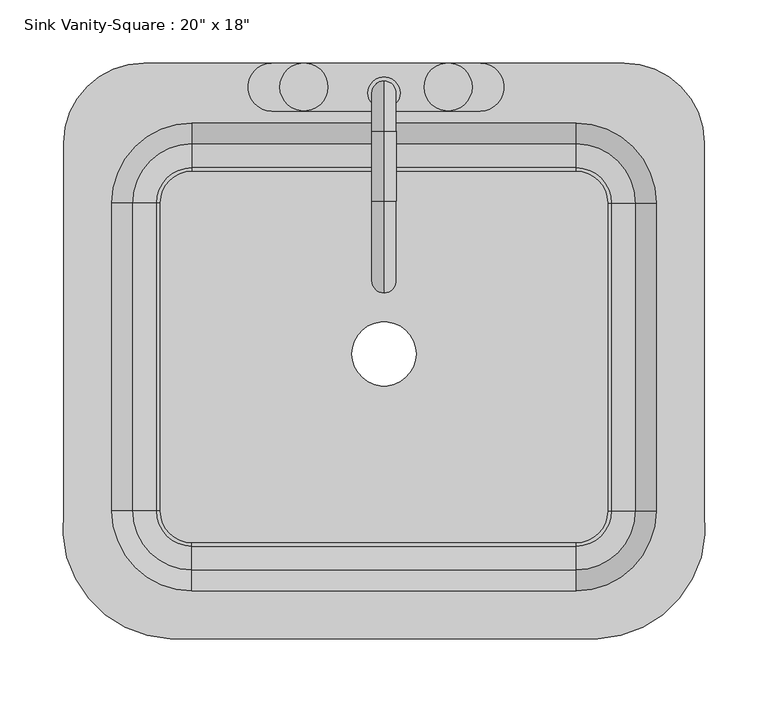
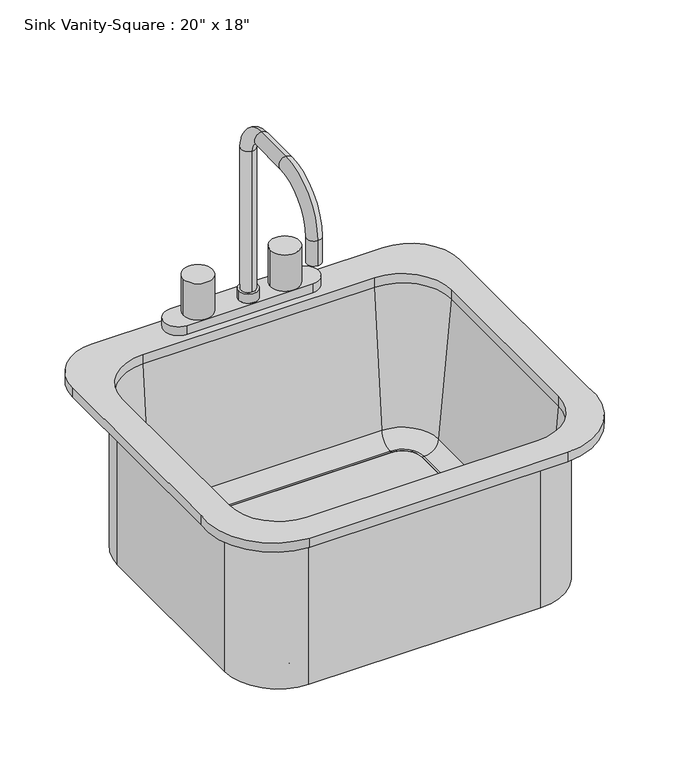
"""IFC4 building model written with IfcOpenShell, lengths in millimetres: flow terminal geometry."""

from ifc_helpers import new_model, si_unit, point, frame, frame_2d, origin, place, context, project, spatial, polyline, circle_curve, ellipse_curve, trimmed, segment, composite_curve, outline, extrude, source, transform, mapped, element, save
from ifc_brep_helpers import plane_surface, cylinder_surface, revolved_surface, advanced_brep


def flow_terminal_62a433f7(model_context):
    return source(origin(), model_context, "Body", "SolidModel", [
        advanced_brep(
        [(-153.9606923, -277.0545989, 800.1), (185.3391735, -277.0545989, 800.1), (269.6892406, -175.4545989, 800.1), (269.6892406, 116.6454011, 800.1), (206.1892406, 180.1454011, 800.1), (-174.8107593, 180.1454011, 800.1), (-238.3107593, 116.6454011, 800.1), (-238.3107593, -175.4545982, 800.1), (168.0892406, 132.5204011, 800.1), (231.5892406, 69.0204011, 800.1), (231.5892406, -175.4545989, 800.1), (168.0892406, -238.9545989, 800.1), (-136.7107594, -238.9545989, 800.1), (-200.2107594, -175.4545989, 800.1), (-200.2107594, 69.0204011, 800.1), (-136.7107594, 132.5204011, 800.1), (-153.9606923, -277.0545989, 787.4), (-238.3107593, -175.4545982, 787.4), (-238.3107593, 116.6454011, 787.4), (-174.8107593, 180.1454011, 787.4), (206.1892406, 180.1454011, 787.4), (269.6892406, 116.6454011, 787.4), (269.6892406, -175.4545989, 787.4), (185.3391735, -277.0545989, 787.4), (237.9392406, 69.0204011, 787.4), (168.0892406, 138.8704011, 787.4), (-136.7107594, 138.8704011, 787.4), (-206.5607594, 69.0204011, 787.4), (-206.5607594, -175.4545989, 787.4), (-136.7107594, -245.3045989, 787.4), (168.0892406, -245.3045989, 787.4), (237.9392406, -175.4545989, 787.4), (168.0892406, 132.5204011, 787.4), (231.5892406, 69.0204011, 787.4), (231.5892406, -175.4545989, 787.4), (168.0892406, -238.9545989, 787.4), (-136.7107594, -238.9545989, 787.4), (-200.2107594, -175.4545989, 787.4), (-200.2107594, 69.0204011, 787.4), (-136.7107594, 132.5204011, 787.4), (237.9392406, 69.0204011, 571.5), (168.0892406, 138.8704011, 571.5), (193.4892406, 69.0204011, 571.5), (168.0892406, 94.4204011, 571.5), (193.4892406, 69.0204011, 581.025), (168.0892406, 94.4204011, 581.025), (196.0776588, 69.0204011, 581.025), (168.0892406, 97.0088193, 581.025), (215.0551678, 69.0204011, 598.4146831), (168.0892406, 115.9863283, 598.4146831), (237.9392406, -175.4545989, 571.5), (193.4892406, -175.4545989, 571.5), (193.4892406, -175.4545989, 581.025), (196.0776588, -175.4545989, 581.025), (215.0551678, -175.4545989, 598.4146831), (168.0892406, -245.3045989, 571.5), (168.0892406, -200.8545989, 571.5), (168.0892406, -200.8545989, 581.025), (168.0892406, -203.4430171, 581.025), (168.0892406, -222.4205261, 598.4146831), (-136.7107594, -245.3045989, 571.5), (-136.7107594, -200.8545989, 571.5), (-136.7107594, -200.8545989, 581.025), (-136.7107594, -203.4430171, 581.025), (-136.7107594, -222.4205261, 598.4146831), (-206.5607594, -175.4545989, 571.5), (-162.1107594, -175.4545989, 571.5), (-162.1107594, -175.4545989, 581.025), (-164.6991776, -175.4545989, 581.025), (-183.6766866, -175.4545989, 598.4146831), (-206.5607594, 69.0204011, 571.5), (-162.1107594, 69.0204011, 571.5), (-162.1107594, 69.0204011, 581.025), (-164.6991776, 69.0204011, 581.025), (-183.6766866, 69.0204011, 598.4146831), (-136.7107594, 138.8704011, 571.5), (-136.7107594, 94.4204011, 571.5), (-136.7107594, 94.4204011, 581.025), (-136.7107594, 97.0088193, 581.025), (-136.7107594, 115.9863283, 598.4146831)],
        [
            (0, 1),
            (1, 2, circle_curve(frame((181.5319557, -188.0793432, 800.1), z_axis=(0.0, 0.0, 1.0), x_axis=(1.0, 0.0, 0.0)), 89.0566732)),
            (2, 3),
            (3, 4, circle_curve(frame((206.1892406, 116.6454011, 800.1), z_axis=(0.0, 0.0, 1.0), x_axis=(1.0, 0.0, 0.0)), 63.5)),
            (4, 5),
            (5, 6, circle_curve(frame((-174.8107593, 116.6454011, 800.1), z_axis=(0.0, 0.0, 1.0), x_axis=(1.0, 0.0, 0.0)), 63.5)),
            (6, 7),
            (7, 0, circle_curve(frame((-150.1534746, -188.0793432, 800.1), z_axis=(0.0, 0.0, 1.0), x_axis=(1.0, 0.0, 0.0)), 89.0566732)),
            (8, 9, circle_curve(frame((168.0892406, 69.0204011, 800.1), z_axis=(0.0, 0.0, -1.0), x_axis=(1.0, 0.0, 0.0)), 63.5)),
            (9, 10),
            (10, 11, circle_curve(frame((168.0892406, -175.4545989, 800.1), z_axis=(0.0, 0.0, -1.0), x_axis=(1.0, 0.0, 0.0)), 63.5)),
            (11, 12),
            (12, 13, circle_curve(frame((-136.7107594, -175.4545989, 800.1), z_axis=(0.0, 0.0, -1.0), x_axis=(1.0, 0.0, 0.0)), 63.5)),
            (13, 14),
            (14, 15, circle_curve(frame((-136.7107594, 69.0204011, 800.1), z_axis=(0.0, 0.0, -1.0), x_axis=(1.0, 0.0, 0.0)), 63.5)),
            (15, 8),
            (16, 17, circle_curve(frame((-150.1534746, -188.0793432, 787.4), z_axis=(0.0, 0.0, -1.0), x_axis=(1.0, 0.0, 0.0)), 89.0566732)),
            (17, 18),
            (18, 19, circle_curve(frame((-174.8107593, 116.6454011, 787.4), z_axis=(0.0, 0.0, -1.0), x_axis=(1.0, 0.0, 0.0)), 63.5)),
            (19, 20),
            (20, 21, circle_curve(frame((206.1892406, 116.6454011, 787.4), z_axis=(0.0, 0.0, -1.0), x_axis=(1.0, 0.0, 0.0)), 63.5)),
            (21, 22),
            (22, 23, circle_curve(frame((181.5319557, -188.0793432, 787.4), z_axis=(0.0, 0.0, -1.0), x_axis=(1.0, 0.0, 0.0)), 89.0566732)),
            (23, 16),
            (24, 25, circle_curve(frame((168.0892406, 69.0204011, 787.4), z_axis=(0.0, 0.0, 1.0), x_axis=(0.0, 1.0, 0.0)), 69.85)),
            (25, 26),
            (26, 27, circle_curve(frame((-136.7107594, 69.0204011, 787.4), z_axis=(0.0, 0.0, 1.0), x_axis=(-1.0, 0.0, 0.0)), 69.85)),
            (27, 28),
            (28, 29, circle_curve(frame((-136.7107594, -175.4545989, 787.4), z_axis=(0.0, 0.0, 1.0), x_axis=(0.0, -1.0, 0.0)), 69.85)),
            (29, 30),
            (30, 31, circle_curve(frame((168.0892406, -175.4545989, 787.4), z_axis=(0.0, 0.0, 1.0), x_axis=(1.0, 0.0, 0.0)), 69.85)),
            (31, 24),
            (0, 16),
            (23, 1),
            (22, 2),
            (21, 3),
            (20, 4),
            (19, 5),
            (18, 6),
            (17, 7),
            (8, 32),
            (32, 33, circle_curve(frame((168.0892406, 69.0204011, 787.4), z_axis=(0.0, 0.0, -1.0), x_axis=(1.0, 0.0, 0.0)), 63.5)),
            (33, 9),
            (33, 34),
            (34, 10),
            (34, 35, circle_curve(frame((168.0892406, -175.4545989, 787.4), z_axis=(0.0, 0.0, -1.0), x_axis=(1.0, 0.0, 0.0)), 63.5)),
            (35, 11),
            (35, 36),
            (36, 12),
            (36, 37, circle_curve(frame((-136.7107594, -175.4545989, 787.4), z_axis=(0.0, 0.0, -1.0), x_axis=(1.0, 0.0, 0.0)), 63.5)),
            (37, 13),
            (37, 38),
            (38, 14),
            (38, 39, circle_curve(frame((-136.7107594, 69.0204011, 787.4), z_axis=(0.0, 0.0, -1.0), x_axis=(1.0, 0.0, 0.0)), 63.5)),
            (39, 15),
            (39, 32),
            (40, 41, circle_curve(frame((168.0892406, 69.0204011, 571.5), z_axis=(0.0, 0.0, 1.0), x_axis=(0.0, 1.0, 0.0)), 69.85)),
            (41, 25),
            (24, 40),
            (40, 42),
            (42, 43, circle_curve(frame((168.0892406, 69.0204011, 571.5), z_axis=(0.0, 0.0, 1.0), x_axis=(0.0, 1.0, 0.0)), 25.4)),
            (43, 41),
            (42, 44),
            (44, 45, circle_curve(frame((168.0892406, 69.0204011, 581.025), z_axis=(0.0, 0.0, 1.0), x_axis=(0.0, 1.0, 0.0)), 25.4)),
            (45, 43),
            (44, 46),
            (46, 47, circle_curve(frame((168.0892406, 69.0204011, 581.025), z_axis=(0.0, 0.0, 1.0), x_axis=(0.0, 1.0, 0.0)), 27.9884182)),
            (47, 45),
            (46, 48, circle_curve(frame((196.0776588, 69.0204011, 600.075), z_axis=(0.0, -1.0, 0.0), x_axis=(1.0, 0.0, 0.0)), 19.05)),
            (48, 49, circle_curve(frame((168.0892406, 69.0204011, 598.4146831), z_axis=(0.0, 0.0, 1.0), x_axis=(0.0, 1.0, 0.0)), 46.9659272)),
            (49, 47, circle_curve(frame((168.0892406, 97.0088193, 600.075), z_axis=(-1.0, 0.0, 0.0), x_axis=(0.0, 1.0, 0.0)), 19.05)),
            (48, 33),
            (32, 49),
            (31, 50),
            (50, 40),
            (50, 51),
            (51, 42),
            (51, 52),
            (52, 44),
            (52, 53),
            (53, 46),
            (53, 54, circle_curve(frame((196.0776588, -175.4545989, 600.075), z_axis=(0.0, -1.0, 0.0), x_axis=(1.0, 0.0, 0.0)), 19.05)),
            (54, 48),
            (54, 34),
            (30, 55),
            (55, 50, circle_curve(frame((168.0892406, -175.4545989, 571.5), z_axis=(0.0, 0.0, 1.0), x_axis=(1.0, 0.0, 0.0)), 69.85)),
            (55, 56),
            (56, 51, circle_curve(frame((168.0892406, -175.4545989, 571.5), z_axis=(0.0, 0.0, 1.0), x_axis=(1.0, 0.0, 0.0)), 25.4)),
            (56, 57),
            (57, 52, circle_curve(frame((168.0892406, -175.4545989, 581.025), z_axis=(0.0, 0.0, 1.0), x_axis=(1.0, 0.0, 0.0)), 25.4)),
            (57, 58),
            (58, 53, circle_curve(frame((168.0892406, -175.4545989, 581.025), z_axis=(0.0, 0.0, 1.0), x_axis=(1.0, 0.0, 0.0)), 27.9884182)),
            (58, 59, circle_curve(frame((168.0892406, -203.4430171, 600.075), z_axis=(-1.0, 0.0, 0.0), x_axis=(0.0, -1.0, 0.0)), 19.05)),
            (59, 54, circle_curve(frame((168.0892406, -175.4545989, 598.4146831), z_axis=(0.0, 0.0, 1.0), x_axis=(1.0, 0.0, 0.0)), 46.9659272)),
            (59, 35),
            (29, 60),
            (60, 55),
            (60, 61),
            (61, 56),
            (61, 62),
            (62, 57),
            (62, 63),
            (63, 58),
            (63, 64, circle_curve(frame((-136.7107594, -203.4430171, 600.075), z_axis=(-1.0, 0.0, 0.0), x_axis=(0.0, -1.0, 0.0)), 19.05)),
            (64, 59),
            (64, 36),
            (28, 65),
            (65, 60, circle_curve(frame((-136.7107594, -175.4545989, 571.5), z_axis=(0.0, 0.0, 1.0), x_axis=(0.0, -1.0, 0.0)), 69.85)),
            (65, 66),
            (66, 61, circle_curve(frame((-136.7107594, -175.4545989, 571.5), z_axis=(0.0, 0.0, 1.0), x_axis=(0.0, -1.0, 0.0)), 25.4)),
            (66, 67),
            (67, 62, circle_curve(frame((-136.7107594, -175.4545989, 581.025), z_axis=(0.0, 0.0, 1.0), x_axis=(0.0, -1.0, 0.0)), 25.4)),
            (67, 68),
            (68, 63, circle_curve(frame((-136.7107594, -175.4545989, 581.025), z_axis=(0.0, 0.0, 1.0), x_axis=(0.0, -1.0, 0.0)), 27.9884182)),
            (68, 69, circle_curve(frame((-164.6991776, -175.4545989, 600.075), z_axis=(0.0, 1.0, 0.0), x_axis=(-1.0, 0.0, 0.0)), 19.05)),
            (69, 64, circle_curve(frame((-136.7107594, -175.4545989, 598.4146831), z_axis=(0.0, 0.0, 1.0), x_axis=(0.0, -1.0, 0.0)), 46.9659272)),
            (69, 37),
            (27, 70),
            (70, 65),
            (70, 71),
            (71, 66),
            (71, 72),
            (72, 67),
            (72, 73),
            (73, 68),
            (73, 74, circle_curve(frame((-164.6991776, 69.0204011, 600.075), z_axis=(0.0, 1.0, 0.0), x_axis=(-1.0, 0.0, 0.0)), 19.05)),
            (74, 69),
            (74, 38),
            (26, 75),
            (75, 70, circle_curve(frame((-136.7107594, 69.0204011, 571.5), z_axis=(0.0, 0.0, 1.0), x_axis=(-1.0, 0.0, 0.0)), 69.85)),
            (75, 76),
            (76, 71, circle_curve(frame((-136.7107594, 69.0204011, 571.5), z_axis=(0.0, 0.0, 1.0), x_axis=(-1.0, 0.0, 0.0)), 25.4)),
            (76, 77),
            (77, 72, circle_curve(frame((-136.7107594, 69.0204011, 581.025), z_axis=(0.0, 0.0, 1.0), x_axis=(-1.0, 0.0, 0.0)), 25.4)),
            (77, 78),
            (78, 73, circle_curve(frame((-136.7107594, 69.0204011, 581.025), z_axis=(0.0, 0.0, 1.0), x_axis=(-1.0, 0.0, 0.0)), 27.9884182)),
            (78, 79, circle_curve(frame((-136.7107594, 97.0088193, 600.075), z_axis=(1.0, 0.0, 0.0), x_axis=(0.0, 1.0, 0.0)), 19.05)),
            (79, 74, circle_curve(frame((-136.7107594, 69.0204011, 598.4146831), z_axis=(0.0, 0.0, 1.0), x_axis=(-1.0, 0.0, 0.0)), 46.9659272)),
            (79, 39),
            (41, 75),
            (43, 76),
            (45, 77),
            (47, 78),
            (49, 79),
        ],
        [
            plane_surface(frame((185.3391735, -277.0545989, 800.1), z_axis=(0.0, 0.0, 1.0), x_axis=(1.0, 0.0, 0.0))),
            plane_surface(frame((185.3391735, -277.0545989, 787.4), z_axis=(0.0, 0.0, -1.0), x_axis=(-1.0, 0.0, 0.0))),
            plane_surface(frame((-153.9606923, -277.0545989, 800.1), z_axis=(0.0, -1.0, 0.0), x_axis=(0.0, 0.0, -1.0))),
            cylinder_surface(frame((181.5319557, -188.0793432, 787.4), z_axis=(0.0, 0.0, 1.0), x_axis=(1.0, 0.0, 0.0)), 89.0566732),
            plane_surface(frame((269.6892406, -175.4545989, 800.1), z_axis=(1.0, 0.0, 0.0), x_axis=(0.0, 0.0, -1.0))),
            cylinder_surface(frame((206.1892406, 116.6454011, 787.4), z_axis=(0.0, 0.0, 1.0), x_axis=(1.0, 0.0, 0.0)), 63.5),
            plane_surface(frame((206.1892406, 180.1454011, 800.1), z_axis=(0.0, 1.0, 0.0), x_axis=(0.0, 0.0, -1.0))),
            cylinder_surface(frame((-174.8107593, 116.6454011, 787.4), z_axis=(0.0, 0.0, 1.0), x_axis=(1.0, 0.0, 0.0)), 63.5),
            plane_surface(frame((-238.3107593, 116.6454011, 800.1), z_axis=(-1.0, 0.0, 0.0), x_axis=(0.0, 0.0, -1.0))),
            cylinder_surface(frame((-150.1534746, -188.0793432, 787.4), z_axis=(0.0, 0.0, 1.0), x_axis=(1.0, 0.0, 0.0)), 89.0566732),
            revolved_surface(polyline([(231.5892406, 69.0204011, 787.4), (231.5892406, 69.0204011, 800.1)]), (168.0892406, 69.0204011, 0.0), (0.0, 0.0, -1.0)),
            plane_surface(frame((231.5892406, 69.0204011, 800.1), z_axis=(-1.0, 0.0, 0.0), x_axis=(0.0, 0.0, -1.0))),
            revolved_surface(polyline([(231.5892406, -175.4545989, 787.4), (231.5892406, -175.4545989, 800.1)]), (168.0892406, -175.4545989, 0.0), (0.0, 0.0, -1.0)),
            plane_surface(frame((168.0892406, -238.9545989, 800.1), z_axis=(0.0, 1.0, 0.0), x_axis=(0.0, 0.0, -1.0))),
            revolved_surface(polyline([(-73.2107594, -175.4545989, 787.4), (-73.2107594, -175.4545989, 800.1)]), (-136.7107594, -175.4545989, 0.0), (0.0, 0.0, -1.0)),
            plane_surface(frame((-200.2107594, -175.4545989, 800.1), z_axis=(1.0, 0.0, 0.0), x_axis=(0.0, 0.0, -1.0))),
            revolved_surface(polyline([(-73.2107594, 69.0204011, 787.4), (-73.2107594, 69.0204011, 800.1)]), (-136.7107594, 69.0204011, 0.0), (0.0, 0.0, -1.0)),
            plane_surface(frame((-136.7107594, 132.5204011, 800.1), z_axis=(0.0, -1.0, 0.0), x_axis=(0.0, 0.0, -1.0))),
            cylinder_surface(frame((168.0892406, 69.0204011, 0.0), z_axis=(0.0, 0.0, -1.0), x_axis=(0.0, 1.0, 0.0)), 69.85),
            plane_surface(frame((168.0892406, 69.0204011, 571.5), z_axis=(0.0, 0.0, -1.0), x_axis=(0.0, 1.0, 0.0))),
            revolved_surface(polyline([(168.0892406, 94.42040109999999, 571.5), (168.0892406, 94.42040109999999, 581.025)]), (168.0892406, 69.0204011, 0.0), (0.0, 0.0, -1.0)),
            plane_surface(frame((168.0892406, 69.0204011, 581.025), z_axis=(0.0, 0.0, 1.0), x_axis=(0.0, 1.0, 0.0))),
            revolved_surface(trimmed(ellipse_curve(frame((168.0892406, 97.0088193, 600.075), z_axis=(1.0, 0.0, 0.0), x_axis=(0.0, 1.0, 0.0)), 19.05, 19.05), [point((168.0892406, 97.0088193, 581.025))], [point((168.0892406, 115.9863283, 598.4146831))], True, "CARTESIAN"), (168.0892406, 69.0204011, 0.0), (0.0, 0.0, -1.0)),
            revolved_surface(polyline([(168.0892406, 115.9863283, 598.4146831), (168.0892406, 132.5204011, 787.4)]), (168.0892406, 69.0204011, 0.0), (0.0, 0.0, -1.0)),
            plane_surface(frame((237.9392406, 69.0204011, 787.4), z_axis=(1.0, 0.0, 0.0), x_axis=(0.0, -1.0, 0.0))),
            plane_surface(frame((237.9392406, 69.0204011, 571.5), z_axis=(0.0, 0.0, -1.0), x_axis=(0.0, -1.0, 0.0))),
            plane_surface(frame((193.4892406, 69.0204011, 571.5), z_axis=(-1.0, 0.0, 0.0), x_axis=(0.0, -1.0, 0.0))),
            plane_surface(frame((193.4892406, 69.0204011, 581.025), z_axis=(0.0, 0.0, 1.0), x_axis=(0.0, -1.0, 0.0))),
            revolved_surface(polyline([(215.1276588, -175.4545989, 600.075), (215.1276588, 69.0204011, 600.075)]), (196.0776588, 69.0204011, 600.075), (0.0, -1.0, 0.0)),
            plane_surface(frame((215.0551678, 69.0204011, 598.4146831), z_axis=(-0.9961946980917442, 0.0, 0.08715574274767397), x_axis=(0.0, -1.0, 0.0))),
            cylinder_surface(frame((168.0892406, -175.4545989, 0.0), z_axis=(0.0, 0.0, -1.0), x_axis=(1.0, 0.0, 0.0)), 69.85),
            plane_surface(frame((168.0892406, -175.4545989, 571.5), z_axis=(0.0, 0.0, -1.0), x_axis=(1.0, 0.0, 0.0))),
            revolved_surface(polyline([(193.48924060000002, -175.4545989, 571.5), (193.48924060000002, -175.4545989, 581.025)]), (168.0892406, -175.4545989, 0.0), (0.0, 0.0, -1.0)),
            plane_surface(frame((168.0892406, -175.4545989, 581.025), z_axis=(0.0, 0.0, 1.0), x_axis=(1.0, 0.0, 0.0))),
            revolved_surface(trimmed(ellipse_curve(frame((196.0776588, -175.4545989, 600.075), z_axis=(0.0, -1.0, 0.0), x_axis=(1.0, 0.0, 0.0)), 19.05, 19.05), [point((196.0776588, -175.4545989, 581.025))], [point((215.0551678, -175.4545989, 598.4146831))], True, "CARTESIAN"), (168.0892406, -175.4545989, 0.0), (0.0, 0.0, -1.0)),
            revolved_surface(polyline([(215.0551678, -175.4545989, 598.4146831), (231.5892406, -175.4545989, 787.4)]), (168.0892406, -175.4545989, 0.0), (0.0, 0.0, -1.0)),
            plane_surface(frame((168.0892406, -245.3045989, 787.4), z_axis=(0.0, -1.0, 0.0), x_axis=(-1.0, 0.0, 0.0))),
            plane_surface(frame((168.0892406, -245.3045989, 571.5), z_axis=(0.0, 0.0, -1.0), x_axis=(-1.0, 0.0, 0.0))),
            plane_surface(frame((168.0892406, -200.8545989, 571.5), z_axis=(0.0, 1.0, 0.0), x_axis=(-1.0, 0.0, 0.0))),
            plane_surface(frame((168.0892406, -200.8545989, 581.025), z_axis=(0.0, 0.0, 1.0), x_axis=(-1.0, 0.0, 0.0))),
            revolved_surface(polyline([(-136.7107594, -222.4930171, 600.075), (168.0892406, -222.4930171, 600.075)]), (168.0892406, -203.4430171, 600.075), (-1.0, 0.0, 0.0)),
            plane_surface(frame((168.0892406, -222.4205261, 598.4146831), z_axis=(0.0, 0.9961946980917442, 0.08715574274767397), x_axis=(-1.0, 0.0, 0.0))),
            cylinder_surface(frame((-136.7107594, -175.4545989, 0.0), z_axis=(0.0, 0.0, -1.0), x_axis=(0.0, -1.0, 0.0)), 69.85),
            plane_surface(frame((-136.7107594, -175.4545989, 571.5), z_axis=(0.0, 0.0, -1.0), x_axis=(0.0, -1.0, 0.0))),
            revolved_surface(polyline([(-136.7107594, -200.8545989, 571.5), (-136.7107594, -200.8545989, 581.025)]), (-136.7107594, -175.4545989, 0.0), (0.0, 0.0, -1.0)),
            plane_surface(frame((-136.7107594, -175.4545989, 581.025), z_axis=(0.0, 0.0, 1.0), x_axis=(0.0, -1.0, 0.0))),
            revolved_surface(trimmed(ellipse_curve(frame((-136.7107594, -203.4430171, 600.075), z_axis=(-1.0, 0.0, 0.0), x_axis=(0.0, -1.0, 0.0)), 19.05, 19.05), [point((-136.7107594, -203.4430171, 581.025))], [point((-136.7107594, -222.4205261, 598.4146831))], True, "CARTESIAN"), (-136.7107594, -175.4545989, 0.0), (0.0, 0.0, -1.0)),
            revolved_surface(polyline([(-136.7107594, -222.4205261, 598.4146831), (-136.7107594, -238.9545989, 787.4)]), (-136.7107594, -175.4545989, 0.0), (0.0, 0.0, -1.0)),
            plane_surface(frame((-206.5607594, -175.4545989, 787.4), z_axis=(-1.0, 0.0, 0.0), x_axis=(0.0, 1.0, 0.0))),
            plane_surface(frame((-206.5607594, -175.4545989, 571.5), z_axis=(0.0, 0.0, -1.0), x_axis=(0.0, 1.0, 0.0))),
            plane_surface(frame((-162.1107594, -175.4545989, 571.5), z_axis=(1.0, 0.0, 0.0), x_axis=(0.0, 1.0, 0.0))),
            plane_surface(frame((-162.1107594, -175.4545989, 581.025), z_axis=(0.0, 0.0, 1.0), x_axis=(0.0, 1.0, 0.0))),
            revolved_surface(polyline([(-183.74917760000002, 69.02040110000002, 600.075), (-183.74917760000002, -175.4545989, 600.075)]), (-164.6991776, -175.4545989, 600.075), (0.0, 1.0, 0.0)),
            plane_surface(frame((-183.6766866, -175.4545989, 598.4146831), z_axis=(0.9961946980917442, 0.0, 0.08715574274767397), x_axis=(0.0, 1.0, 0.0))),
            cylinder_surface(frame((-136.7107594, 69.0204011, 0.0), z_axis=(0.0, 0.0, -1.0), x_axis=(-1.0, 0.0, 0.0)), 69.85),
            plane_surface(frame((-136.7107594, 69.0204011, 571.5), z_axis=(0.0, 0.0, -1.0), x_axis=(-1.0, 0.0, 0.0))),
            revolved_surface(polyline([(-162.1107594, 69.0204011, 571.5), (-162.1107594, 69.0204011, 581.025)]), (-136.7107594, 69.0204011, 0.0), (0.0, 0.0, -1.0)),
            plane_surface(frame((-136.7107594, 69.0204011, 581.025), z_axis=(0.0, 0.0, 1.0), x_axis=(-1.0, 0.0, 0.0))),
            revolved_surface(trimmed(ellipse_curve(frame((-164.6991776, 69.0204011, 600.075), z_axis=(0.0, 1.0, 0.0), x_axis=(-1.0, 0.0, 0.0)), 19.05, 19.05), [point((-164.6991776, 69.0204011, 581.025))], [point((-183.6766866, 69.0204011, 598.4146831))], True, "CARTESIAN"), (-136.7107594, 69.0204011, 0.0), (0.0, 0.0, -1.0)),
            revolved_surface(polyline([(-183.6766866, 69.0204011, 598.4146831), (-200.2107594, 69.0204011, 787.4)]), (-136.7107594, 69.0204011, 0.0), (0.0, 0.0, -1.0)),
            plane_surface(frame((-136.7107594, 138.8704011, 787.4), z_axis=(0.0, 1.0, 0.0), x_axis=(1.0, 0.0, 0.0))),
            plane_surface(frame((-136.7107594, 138.8704011, 571.5), z_axis=(0.0, 0.0, -1.0), x_axis=(1.0, 0.0, 0.0))),
            plane_surface(frame((-136.7107594, 94.4204011, 571.5), z_axis=(0.0, -1.0, 0.0), x_axis=(1.0, 0.0, 0.0))),
            plane_surface(frame((-136.7107594, 94.4204011, 581.025), z_axis=(0.0, 0.0, 1.0), x_axis=(1.0, 0.0, 0.0))),
            revolved_surface(polyline([(168.0892406, 116.0588193, 600.075), (-136.7107594, 116.0588193, 600.075)]), (-136.7107594, 97.0088193, 600.075), (1.0, 0.0, 0.0)),
            plane_surface(frame((-136.7107594, 115.9863283, 598.4146831), z_axis=(0.0, -0.9961946980917442, 0.08715574274767397), x_axis=(1.0, 0.0, 0.0))),
        ],
        [
            (0, [[1, 2, 3, 4, 5, 6, 7, 8], [9, 10, 11, 12, 13, 14, 15, 16]]),
            (1, [[17, 18, 19, 20, 21, 22, 23, 24], [25, 26, 27, 28, 29, 30, 31, 32]]),
            (2, [[-1, 33, -24, 34]]),
            (3, [[-2, -34, -23, 35]]),
            (4, [[-3, -35, -22, 36]]),
            (5, [[-4, -36, -21, 37]]),
            (6, [[-5, -37, -20, 38]]),
            (7, [[-6, -38, -19, 39]]),
            (8, [[-7, -39, -18, 40]]),
            (9, [[-8, -40, -17, -33]]),
            (10, [[-9, 41, 42, 43]]),
            (11, [[-10, -43, 44, 45]]),
            (12, [[-11, -45, 46, 47]]),
            (13, [[-12, -47, 48, 49]]),
            (14, [[-13, -49, 50, 51]]),
            (15, [[-14, -51, 52, 53]]),
            (16, [[-15, -53, 54, 55]]),
            (17, [[-16, -55, 56, -41]]),
            (18, [[57, 58, -25, 59]]),
            (19, [[-57, 60, 61, 62]]),
            (20, [[-61, 63, 64, 65]]),
            (21, [[-64, 66, 67, 68]]),
            (22, [[-67, 69, 70, 71]]),
            (23, [[-70, 72, -42, 73]]),
            (24, [[-59, -32, 74, 75]]),
            (25, [[-60, -75, 76, 77]]),
            (26, [[-63, -77, 78, 79]]),
            (27, [[-66, -79, 80, 81]]),
            (28, [[-69, -81, 82, 83]]),
            (29, [[-72, -83, 84, -44]]),
            (30, [[-74, -31, 85, 86]]),
            (31, [[-76, -86, 87, 88]]),
            (32, [[-78, -88, 89, 90]]),
            (33, [[-80, -90, 91, 92]]),
            (34, [[-82, -92, 93, 94]]),
            (35, [[-84, -94, 95, -46]]),
            (36, [[-85, -30, 96, 97]]),
            (37, [[-87, -97, 98, 99]]),
            (38, [[-89, -99, 100, 101]]),
            (39, [[-91, -101, 102, 103]]),
            (40, [[-93, -103, 104, 105]]),
            (41, [[-95, -105, 106, -48]]),
            (42, [[-96, -29, 107, 108]]),
            (43, [[-98, -108, 109, 110]]),
            (44, [[-100, -110, 111, 112]]),
            (45, [[-102, -112, 113, 114]]),
            (46, [[-104, -114, 115, 116]]),
            (47, [[-106, -116, 117, -50]]),
            (48, [[-107, -28, 118, 119]]),
            (49, [[-109, -119, 120, 121]]),
            (50, [[-111, -121, 122, 123]]),
            (51, [[-113, -123, 124, 125]]),
            (52, [[-115, -125, 126, 127]]),
            (53, [[-117, -127, 128, -52]]),
            (54, [[-118, -27, 129, 130]]),
            (55, [[-120, -130, 131, 132]]),
            (56, [[-122, -132, 133, 134]]),
            (57, [[-124, -134, 135, 136]]),
            (58, [[-126, -136, 137, 138]]),
            (59, [[-128, -138, 139, -54]]),
            (60, [[-58, 140, -129, -26]]),
            (61, [[-62, 141, -131, -140]]),
            (62, [[-65, 142, -133, -141]]),
            (63, [[-68, 143, -135, -142]]),
            (64, [[-71, 144, -137, -143]]),
            (65, [[-73, -56, -139, -144]]),
        ],
    ),
        advanced_brep(
        [(91.8892406, 180.1454011, 800.1), (91.8892406, 142.0454011, 800.1), (-73.2107594, 142.0454011, 800.1), (-73.2107594, 180.1454011, 800.1), (15.6892406, 165.8579011, 1020.7625), (15.6892406, 146.8079011, 1020.7625), (15.6892406, 146.8079011, 825.5), (15.6892406, 165.8579011, 825.5), (15.6892406, 126.1704011, 1060.45), (15.6892406, 126.1704011, 1041.4), (15.6892406, 70.6079011, 1060.45), (15.6892406, 70.6079011, 1041.4), (15.6892406, -2.4170989, 987.425), (15.6892406, 16.6329011, 987.425), (15.6892406, -2.4170989, 952.5), (15.6892406, 16.6329011, 952.5), (2.9892406, 156.3329011, 825.5), (28.3892406, 156.3329011, 825.5), (2.9892406, 156.3329011, 812.8), (28.3892406, 156.3329011, 812.8), (91.8892406, 180.1454011, 812.8), (-73.2107594, 180.1454011, 812.8), (-73.2107594, 142.0454011, 812.8), (91.8892406, 142.0454011, 812.8)],
        [
            (0, 1, circle_curve(frame((91.8892406, 161.0954011, 800.1), z_axis=(0.0, 0.0, -1.0), x_axis=(1.0, 0.0, 0.0)), 19.05)),
            (1, 2),
            (2, 3, circle_curve(frame((-73.2107594, 161.0954011, 800.1), z_axis=(0.0, 0.0, -1.0), x_axis=(1.0, 0.0, 0.0)), 19.05)),
            (3, 0),
            (4, 5, circle_curve(frame((15.6892406, 156.3329011, 1020.7625), z_axis=(0.0, 0.0, -1.0), x_axis=(0.0, -1.0, 0.0)), 9.525)),
            (5, 6),
            (6, 7, circle_curve(frame((15.6892406, 156.3329011, 825.5), z_axis=(0.0, 0.0, 1.0), x_axis=(0.0, -1.0, 0.0)), 9.525)),
            (7, 4),
            (5, 4, circle_curve(frame((15.6892406, 156.3329011, 1020.7625), z_axis=(0.0, 0.0, -1.0), x_axis=(0.0, -1.0, 0.0)), 9.525)),
            (7, 6, circle_curve(frame((15.6892406, 156.3329011, 825.5), z_axis=(0.0, 0.0, 1.0), x_axis=(0.0, -1.0, 0.0)), 9.525)),
            (4, 8, circle_curve(frame((15.6892406, 126.1704011, 1020.7625), z_axis=(1.0, 0.0, 0.0), x_axis=(0.0, 1.0, 0.0)), 39.6875)),
            (8, 9, circle_curve(frame((15.6892406, 126.1704011, 1050.925), z_axis=(0.0, 1.0, 0.0), x_axis=(0.0, 0.0, -1.0)), 9.525)),
            (9, 5, circle_curve(frame((15.6892406, 126.1704011, 1020.7625), z_axis=(-1.0, 0.0, 0.0), x_axis=(0.0, 1.0, 0.0)), 20.6375)),
            (9, 8, circle_curve(frame((15.6892406, 126.1704011, 1050.925), z_axis=(0.0, 1.0, 0.0), x_axis=(0.0, 0.0, -1.0)), 9.525)),
            (8, 10),
            (10, 11, circle_curve(frame((15.6892406, 70.6079011, 1050.925), z_axis=(0.0, 1.0, 0.0), x_axis=(0.0, 0.0, -1.0)), 9.525)),
            (11, 9),
            (11, 10, circle_curve(frame((15.6892406, 70.6079011, 1050.925), z_axis=(0.0, 1.0, 0.0), x_axis=(0.0, 0.0, -1.0)), 9.525)),
            (10, 12, circle_curve(frame((15.6892406, 70.6079011, 987.425), z_axis=(1.0, 0.0, 0.0), x_axis=(0.0, 0.0, 1.0)), 73.025)),
            (12, 13, circle_curve(frame((15.6892406, 7.1079011, 987.425), z_axis=(0.0, 0.0, 1.0), x_axis=(0.0, 1.0, 0.0)), 9.525)),
            (13, 11, circle_curve(frame((15.6892406, 70.6079011, 987.425), z_axis=(-1.0, 0.0, 0.0), x_axis=(0.0, 0.0, 1.0)), 53.975)),
            (13, 12, circle_curve(frame((15.6892406, 7.1079011, 987.425), z_axis=(0.0, 0.0, 1.0), x_axis=(0.0, 1.0, 0.0)), 9.525)),
            (14, 15, circle_curve(frame((15.6892406, 7.1079011, 952.5), z_axis=(0.0, 0.0, -1.0), x_axis=(0.0, 1.0, 0.0)), 9.525)),
            (15, 14, circle_curve(frame((15.6892406, 7.1079011, 952.5), z_axis=(0.0, 0.0, -1.0), x_axis=(0.0, 1.0, 0.0)), 9.525)),
            (12, 14),
            (15, 13),
            (16, 17, circle_curve(frame((15.6892406, 156.3329011, 825.5), z_axis=(0.0, 0.0, 1.0), x_axis=(1.0, 0.0, 0.0)), 12.7)),
            (17, 16, circle_curve(frame((15.6892406, 156.3329011, 825.5), z_axis=(0.0, 0.0, 1.0), x_axis=(1.0, 0.0, 0.0)), 12.7)),
            (16, 18),
            (18, 19, circle_curve(frame((15.6892406, 156.3329011, 812.8), z_axis=(0.0, 0.0, 1.0), x_axis=(1.0, 0.0, 0.0)), 12.7)),
            (19, 17),
            (19, 18, circle_curve(frame((15.6892406, 156.3329011, 812.8), z_axis=(0.0, 0.0, 1.0), x_axis=(1.0, 0.0, 0.0)), 12.7)),
            (20, 21),
            (21, 22, circle_curve(frame((-73.2107594, 161.0954011, 812.8), z_axis=(0.0, 0.0, 1.0), x_axis=(1.0, 0.0, 0.0)), 19.05)),
            (22, 23),
            (23, 20, circle_curve(frame((91.8892406, 161.0954011, 812.8), z_axis=(0.0, 0.0, 1.0), x_axis=(1.0, 0.0, 0.0)), 19.05)),
            (20, 0),
            (3, 21),
            (2, 22),
            (1, 23),
        ],
        [
            plane_surface(frame((15.6892406, 146.8079011, 800.1), z_axis=(0.0, 0.0, -1.0), x_axis=(1.0, 0.0, 0.0))),
            cylinder_surface(frame((15.6892406, 156.3329011, 800.1), z_axis=(0.0, 0.0, -1.0), x_axis=(0.0, -1.0, 0.0)), 9.525),
            revolved_surface(trimmed(ellipse_curve(frame((15.6892406, 156.3329011, 1020.7625), z_axis=(0.0, 0.0, -1.0), x_axis=(0.0, -1.0, 0.0)), 9.525, 9.525), [point((15.6892406, 165.8579011, 1020.7625))], [point((15.6892406, 146.8079011, 1020.7625))], True, "CARTESIAN"), (15.6892406, 126.1704011, 1020.7625), (1.0, 0.0, 0.0)),
            revolved_surface(trimmed(ellipse_curve(frame((15.6892406, 156.3329011, 1020.7625), z_axis=(0.0, 0.0, -1.0), x_axis=(0.0, -1.0, 0.0)), 9.525, 9.525), [point((15.6892406, 146.8079011, 1020.7625))], [point((15.6892406, 165.8579011, 1020.7625))], True, "CARTESIAN"), (15.6892406, 126.1704011, 1020.7625), (1.0, 0.0, 0.0)),
            cylinder_surface(frame((15.6892406, 126.1704011, 1050.925), z_axis=(0.0, 1.0, 0.0), x_axis=(0.0, 0.0, -1.0)), 9.525),
            revolved_surface(trimmed(ellipse_curve(frame((15.6892406, 70.6079011, 1050.925), z_axis=(0.0, 1.0, 0.0), x_axis=(0.0, 0.0, -1.0)), 9.525, 9.525), [point((15.6892406, 70.6079011, 1060.45))], [point((15.6892406, 70.6079011, 1041.4))], True, "CARTESIAN"), (15.6892406, 70.6079011, 987.425), (1.0, 0.0, 0.0)),
            revolved_surface(trimmed(ellipse_curve(frame((15.6892406, 70.6079011, 1050.925), z_axis=(0.0, 1.0, 0.0), x_axis=(0.0, 0.0, -1.0)), 9.525, 9.525), [point((15.6892406, 70.6079011, 1041.4))], [point((15.6892406, 70.6079011, 1060.45))], True, "CARTESIAN"), (15.6892406, 70.6079011, 987.425), (1.0, 0.0, 0.0)),
            plane_surface(frame((15.6892406, -2.4170989, 952.5), z_axis=(0.0, 0.0, -1.0), x_axis=(-1.0, 0.0, 0.0))),
            cylinder_surface(frame((15.6892406, 7.1079011, 987.425), z_axis=(0.0, 0.0, 1.0), x_axis=(0.0, 1.0, 0.0)), 9.525),
            plane_surface(frame((28.3892406, 156.3329011, 825.5), z_axis=(0.0, 0.0, 1.0), x_axis=(0.0, 1.0, 0.0))),
            cylinder_surface(frame((15.6892406, 156.3329011, 812.8), z_axis=(0.0, 0.0, 1.0), x_axis=(1.0, 0.0, 0.0)), 12.7),
            plane_surface(frame((-73.2107594, 180.1454011, 812.8), z_axis=(0.0, 0.0, 1.0), x_axis=(-1.0, 0.0, 0.0))),
            plane_surface(frame((91.8892406, 180.1454011, 812.8), z_axis=(0.0, 1.0, 0.0), x_axis=(0.0, 0.0, -1.0))),
            cylinder_surface(frame((-73.2107594, 161.0954011, 800.1), z_axis=(0.0, 0.0, 1.0), x_axis=(1.0, 0.0, 0.0)), 19.05),
            plane_surface(frame((-73.2107594, 142.0454011, 812.8), z_axis=(0.0, -1.0, 0.0), x_axis=(0.0, 0.0, -1.0))),
            cylinder_surface(frame((91.8892406, 161.0954011, 800.1), z_axis=(0.0, 0.0, 1.0), x_axis=(1.0, 0.0, 0.0)), 19.05),
        ],
        [
            (0, [[1, 2, 3, 4]]),
            (1, [[5, 6, 7, 8]]),
            (1, [[9, -8, 10, -6]]),
            (2, [[-5, 11, 12, 13]]),
            (3, [[-9, -13, 14, -11]]),
            (4, [[-12, 15, 16, 17]]),
            (4, [[-14, -17, 18, -15]]),
            (5, [[-16, 19, 20, 21]]),
            (6, [[-18, -21, 22, -19]]),
            (7, [[23, 24]]),
            (8, [[-20, 25, -24, 26]]),
            (8, [[-22, -26, -23, -25]]),
            (9, [[27, 28], [-7, -10]]),
            (10, [[-27, 29, 30, 31]]),
            (10, [[-28, -31, 32, -29]]),
            (11, [[33, 34, 35, 36], [-30, -32]]),
            (12, [[-33, 37, -4, 38]]),
            (13, [[-34, -38, -3, 39]]),
            (14, [[-35, -39, -2, 40]]),
            (15, [[-36, -40, -1, -37]]),
        ],
    ),
        extrude(outline(composite_curve([segment(trimmed(circle_curve(frame_2d((-47.8107594, 161.0954011)), 19.05), [point((-66.8607594, 161.0954011))], [point((-28.7607594, 161.0954011))], False, "CARTESIAN"), True, "CONTINUOUS"), segment(trimmed(circle_curve(frame_2d((-47.8107594, 161.0954011)), 19.05), [point((-28.7607594, 161.0954011))], [point((-66.8607594, 161.0954011))], False, "CARTESIAN"), True, "CONTINUOUS")], self_intersect=False)), frame((0.0, 0.0, 812.8), z_axis=(0.0, 0.0, 1.0), x_axis=(1.0, 0.0, 0.0)), (0.0, 0.0, 1.0), 50.8),
        extrude(outline(composite_curve([segment(trimmed(circle_curve(frame_2d((66.4892406, 161.0954011)), 19.05), [point((47.4392406, 161.0954011))], [point((85.5392406, 161.0954011))], False, "CARTESIAN"), True, "CONTINUOUS"), segment(trimmed(circle_curve(frame_2d((66.4892406, 161.0954011)), 19.05), [point((85.5392406, 161.0954011))], [point((47.4392406, 161.0954011))], False, "CARTESIAN"), True, "CONTINUOUS")], self_intersect=False)), frame((0.0, 0.0, 812.8), z_axis=(0.0, 0.0, 1.0), x_axis=(1.0, 0.0, 0.0)), (0.0, 0.0, 1.0), 50.8),
        extrude(outline(composite_curve([segment(trimmed(circle_curve(frame_2d((168.0892406, 69.0204011)), 25.4), [point((168.0892406, 94.4204011))], [point((193.4892406, 69.0204011))], False, "CARTESIAN"), True, "CONTINUOUS"), segment(polyline([(193.4892406, 69.0204011), (193.4892406, -175.4545989)]), True, "CONTINUOUS"), segment(trimmed(circle_curve(frame_2d((168.0892406, -175.4545989)), 25.4), [point((193.4892406, -175.4545989))], [point((168.0892406, -200.8545989))], False, "CARTESIAN"), True, "CONTINUOUS"), segment(polyline([(168.0892406, -200.8545989), (-136.7107594, -200.8545989)]), True, "CONTINUOUS"), segment(trimmed(circle_curve(frame_2d((-136.7107594, -175.4545989)), 25.4), [point((-136.7107594, -200.8545989))], [point((-162.1107594, -175.4545989))], False, "CARTESIAN"), True, "CONTINUOUS"), segment(polyline([(-162.1107594, -175.4545989), (-162.1107594, 69.0204011)]), True, "CONTINUOUS"), segment(trimmed(circle_curve(frame_2d((-136.7107594, 69.0204011)), 25.4), [point((-162.1107594, 69.0204011))], [point((-136.7107594, 94.4204011))], False, "CARTESIAN"), True, "CONTINUOUS"), segment(polyline([(-136.7107594, 94.4204011), (168.0892406, 94.4204011)]), True, "CONTINUOUS")], self_intersect=False), holes=[composite_curve([segment(trimmed(circle_curve(frame_2d((15.6892406, -50.8)), 25.4), [point((-9.7107594, -50.8))], [point((41.0892406, -50.8))], True, "CARTESIAN"), True, "CONTINUOUS"), segment(trimmed(circle_curve(frame_2d((15.6892406, -50.8)), 25.4), [point((41.0892406, -50.8))], [point((-9.7107594, -50.8))], True, "CARTESIAN"), True, "CONTINUOUS")], self_intersect=False)]), frame((0.0, 0.0, 571.5), z_axis=(0.0, 0.0, 1.0), x_axis=(1.0, 0.0, 0.0)), (0.0, 0.0, 1.0), 9.525),
    ])


if __name__ == "__main__":
    model = new_model("IFC4")
    model_context = context("Model", 3, world=origin())
    ifc_project = project(units=[si_unit("LENGTHUNIT", "METRE", prefix="MILLI")], contexts=[model_context])
    site = spatial("IfcSite", under=ifc_project)
    building = spatial("IfcBuilding", under=site)
    placement = place(None, origin())
    flow_terminal_shape = flow_terminal_62a433f7(model_context)
    element("IfcFlowTerminal", 1, ObjectType="Sink Vanity-Square : 20\" x 18\"", at=placement, inside=building, context=model_context, shape_type="MappedRepresentation", body=[
        mapped(flow_terminal_shape, transform((0.0, 0.0, 0.0), x_axis=(1.0, 0.0, 0.0), y_axis=(0.0, 1.0, 0.0), z_axis=(0.0, 0.0, 1.0))),
    ])
    save(model, "model.ifc")

# Revit data of these elements
# Type "Sink Vanity-Square : 20\" x 18\""
#   Assembly Code = "D2010400"
#   Counter Height = 2' - 7"
#   Depth = 1' - 6"
#   Width = 1' - 8"
#   Basin Material = Porcelain, Linen
#   Faucet Material = Steel, Polished
#   Default Elevation = 0
# Element 1 (IfcFlowTerminal, "Sink Vanity-Square : 20\" x 18\"")
#   Materials on its faces: "Porcelain, Linen", "Steel, Polished"
# Materials
#   "Porcelain, Linen": class "Ceramic", colour RGB 249 239 230, transparency 0, Description = "Porcelain, linen", Cost = 0
#   "Steel, Polished": class "Metal", colour RGB 57 57 57, transparency 0, Description = "Polished steel", Cost = 0
